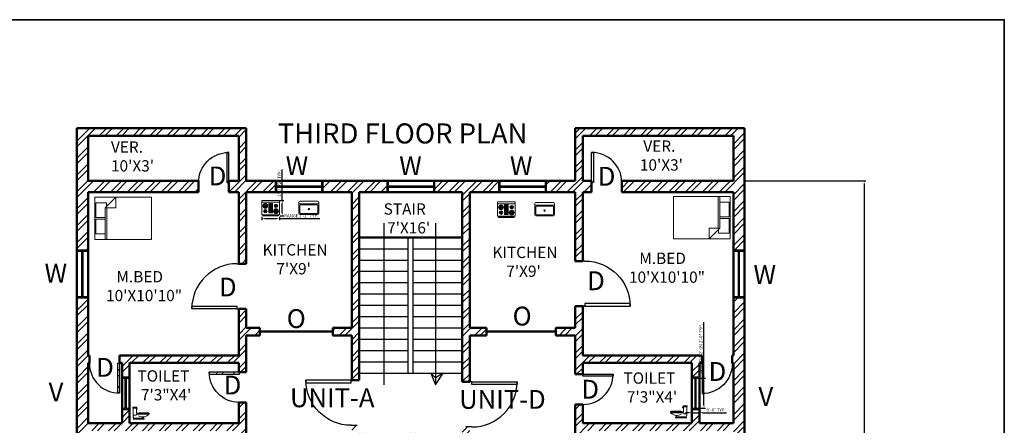
# Model space of a CAD drawing. Units: inches. Extents: x -31842 to -29388, y 18869 to 19743.
# Tile 12 of 12: x -30172 to -29388, y 19420 to 19743. Entities that reach past the tile are written whole.
import ezdxf

# ---------------------------------------------------------------- set-up
doc = ezdxf.new("R2010")
doc.units = ezdxf.units.IN
for name, color, linetype, lineweight in [('A-ANNO-DIMS', 2, 'Continuous', 18), ('A-ANNO-SYMB', 2, 'Continuous', 18), ('A-ANNO-TEXT', 7, 'Continuous', 25), ('A-ANNO-TTLB', 7, 'Continuous', 35), ('A-AREA-IDEN', 3, 'Continuous', 18), ('A-DOOR', 3, 'Continuous', 25), ('A-FLOR-FIXT', 8, 'Continuous', 18), ('A-FLOR-STRS', 7, 'Continuous', 25), ('A-FURN', 8, 'Continuous', 18), ('A-GLAZ', 4, 'Continuous', 25), ('A-WALL', 7, 'Continuous', 50), ('A-WALL-PATT', 8, 'Continuous', 13)]:
    doc.layers.add(name, color=color, linetype=linetype, lineweight=lineweight)
doc.styles.get("Standard").update_dxf_attribs({"font": 'arial.ttf'})
doc.dimstyles.new('ISO-25', dxfattribs={"dimtxt": 2.5, "dimasz": 2.5, "dimexe": 1.25, "dimexo": 0.625, "dimtad": 1, "dimdec": 0, "dimlunit": 3, "dimtxsty": 'Standard', "dimcen": 2.5, "dimadec": 0, "dimazin": 0, "dimtfac": 1, "dimtdec": 0, "dimtmove": 0, "dimatfit": 3, "dimfxl": 1, "dimarcsym": 0})

# ---------------------------------------------------------------- blocks, each defined once
blk = doc.blocks.new('*U8')
for p, q in [((0, 0), (0, -100)), ((750, 0), (750, -100))]:
    blk.add_line(p, q)
blk.add_lwpolyline([(0, 0), (0, 750), (43.75, 750), (43.75, 0)], close=True)
blk.add_arc((0, 0), 750, 0, 90)
blk = doc.blocks.new('Bed - Queen')
for p, q in [((0, -80.00003), (0, 0)), ((0, 0), (59.99999, 0)), ((59.99999, 0), (59.99999, -80.00003)), ((7.99999, -1.2), (28.79998, -1.2)), ((7.99999, -14.4), (7.99999, -1.2)), ((28.79998, -1.2), (28.79998, -14.4)), ((31.19999, -1.2), (51.99999, -1.2)), ((31.19999, -14.4), (31.19999, -1.2)), ((51.99999, -1.2), (51.99999, -16.4)), ((0, -14.4), (44.8, -14.4)), ((44.8, -16.8), (0, -16.8)), ((59.99999, -29.6), (44.8, -14.4)), ((44.8, -14.4), (44.8, -29.6)), ((51.99999, -16.4), (46.79936, -16.4)), ((44.8, -29.6), (59.99999, -29.6)), ((59.99999, -80.00003), (0, -80.00003))]:
    blk.add_line(p, q)
blk = doc.blocks.new('Range-Oven - 30 in top')
for p, q in [((0, -3), (30, -3)), ((12, -6), (18, -6)), ((13, -20), (13, -6)), ((14, -6), (14, -20)), ((15, -20), (15, -6)), ((16, -6), (16, -20)), ((17, -20), (17, -6)), ((6, -24), (6, -25)), ((8, -25), (8, -24)), ((18, -20), (12, -20)), ((22, -25), (22, -24)), ((24, -24), (24, -25))]:
    blk.add_line(p, q)
for points in [[(0, -24), (0, 0), (30, 0), (30, -24)], [(12, -21), (12, -5), (18, -5), (18, -21)], [(2, -26), (2, -25), (28, -25), (28, -26)]]:
    blk.add_lwpolyline(points, close=True)
for centre, radius in [((6, -9), 4), ((6, -9), 3), ((6, -18), 3), ((6, -9), 2), ((6, -18), 2), ((6, -9), 1), ((24, -18), 4), ((24, -9), 3), ((24, -18), 3), ((24, -9), 2), ((24, -18), 2), ((24, -9), 1), ((6, -18), 1), ((24, -18), 1)]:
    blk.add_circle(centre, radius)
blk = doc.blocks.new('Sink-single - 30 in top')
blk.add_line((-15, -3.999996), (15, -3.999996))
for points in [[(-13.5, 0), (13.5, 0)], [(-15, -18.499996), (-15, -1.5)], [(-13.5, -17.499996), (-13.5, -6.499996)], [(-12.5, -5.499996), (12.5, -5.499996)], [(13.5, -6.499996), (13.5, -17.499996)], [(15, -1.5), (15, -18.499996)], [(13.5, -19.999996), (-13.5, -19.999996)], [(12.5, -18.499996), (-12.5, -18.499996)]]:
    blk.add_lwpolyline(points)
for radius in [1, 0.5]:
    blk.add_circle((0, -11.999996), radius)
for centre, radius, start, end in [((-13.5, -1.5), 1.5, 90, 180), ((-12.5, -6.499996), 1, 90, 180), ((12.5, -6.499996), 1, 0, 90), ((13.5, -1.5), 1.5, 0, 90), ((-13.5, -18.499996), 1.5, 180, 270), ((-12.5, -17.499996), 1, 180, 270), ((12.5, -17.499996), 1, 270, 0), ((13.5, -18.499996), 1.5, 270, 0)]:
    blk.add_arc(centre, radius, start, end)
blk = doc.blocks.new('Toilet - side')
for p, q in [((0.5, 5), (0.5, 22)), ((7.5, 22), (7.5, 12)), ((7.5, 21), (9, 21)), ((9, 20), (7.5, 20)), ((9, 21), (9, 20)), ((6, 8), (0.5, 8)), ((22, 2), (2, 2)), ((2, 2), (2, 1)), ((8, 10), (6, 8)), ((7.5, 12), (33, 12)), ((33, 10), (8, 10)), ((32.5, 13), (12, 13)), ((12, 13), (12, 12)), ((21, 4.5), (21, 2)), ((22, 2), (22, 4.5)), ((22, 1), (22, 2)), ((32.5, 12), (32.5, 13)), ((33, 12), (33, 10))]:
    blk.add_line(p, q)
for points in [[(0, 22), (0, 24), (8, 24), (8, 22)], [(1, 0), (1, 1), (23, 1), (23, 0)]]:
    blk.add_lwpolyline(points, close=True)
for centre, radius, start, end in [((3.8, 4.8), 3.26, 175.6013, 237.5288), ((20.3, 20.7), 16.2, 238.1872, 318.7702)]:
    blk.add_arc(centre, radius, start, end)
blk = doc.blocks.new('*D211')
at = {"layer": 'A-ANNO-DIMS', "color": 0, "lineweight": -2, "transparency": 16777216}
for p, q in [((-29593.87, 19614.96), (-29498.06, 19614.96)), ((-29499.31, 19612.46), (-29499.31, 19017.46)), ((-29593.87, 19014.96), (-29498.06, 19014.96))]:
    blk.add_line(p, q, dxfattribs=at)
at = {"layer": 'A-ANNO-DIMS', "color": 0, "transparency": 16777216}
for points in [[(-29499.72, 19612.46), (-29498.89, 19612.46), (-29499.31, 19614.96)], [(-29499.72, 19017.46), (-29498.89, 19017.46), (-29499.31, 19014.96)]]:
    blk.add_solid(points, dxfattribs=at)
at = {"layer": 'Defpoints', "color": 0, "transparency": 16777216}
for p in [(-29594.5, 19614.96), (-29594.5, 19014.96), (-29499.31, 19014.96)]:
    blk.add_point(p, dxfattribs=at)
at = {"layer": 'A-ANNO-DIMS', "color": 0, "transparency": 16777216, "insert": (-29508.1, 19314.96), "char_height": 2.5, "attachment_point": 5, "rotation": 90}
blk.add_mtext("{\\H6.4x;50'}", dxfattribs=at)
blk = doc.blocks.new('WIN-3FT')
for p, q in [((0, 36), (9, 36)), ((4, 0), (4, 36)), ((4.5, 0), (4.5, 36)), ((5, 0), (5, 36)), ((0, 0), (9, 0))]:
    blk.add_line(p, q)
blk = doc.blocks.new('WIN-2FT-B')
for p, q in [((0, 24), (6, 24)), ((2.5, 0), (2.5, 24)), ((3, 0), (3, 24)), ((3.5, 0), (3.5, 24)), ((0, 0), (6, 0))]:
    blk.add_line(p, q)
blk = doc.blocks.new('*D235')
at = {"layer": 'A-ANNO-DIMS', "color": 0, "lineweight": -2, "transparency": 16777216}
for p, q in [((-29979.2, 19586.46), (-29979.2, 19583.71)), ((-29965.04, 19586.46), (-29965.04, 19583.71)), ((-29976.7, 19584.96), (-29967.54, 19584.96)), ((-29965.04, 19584.96), (-29932.79, 19584.96))]:
    blk.add_line(p, q, dxfattribs=at)
at = {"layer": 'A-ANNO-DIMS', "color": 0, "transparency": 16777216}
for points in [[(-29976.7, 19585.38), (-29976.7, 19584.54), (-29979.2, 19584.96)], [(-29967.54, 19585.38), (-29967.54, 19584.54), (-29965.04, 19584.96)]]:
    blk.add_solid(points, dxfattribs=at)
at = {"layer": 'Defpoints', "color": 0, "transparency": 16777216}
for p in [(-29979.2, 19587.08), (-29965.04, 19587.08), (-29965.04, 19584.96)]:
    blk.add_point(p, dxfattribs=at)
at = {"layer": 'A-ANNO-DIMS', "color": 0, "transparency": 16777216, "insert": (-29947.66, 19586.88), "char_height": 2.5, "attachment_point": 5}
blk.add_mtext('RANGE 1\'-2" TYP.', dxfattribs=at)
blk = doc.blocks.new('*D236')
at = {"layer": 'A-ANNO-DIMS', "color": 0, "lineweight": -2, "transparency": 16777216}
for p, q in [((-29962.91, 19599.36), (-29962.91, 19623.94)), ((-29964.41, 19599.36), (-29961.66, 19599.36)), ((-29962.91, 19589.58), (-29962.91, 19596.86)), ((-29964.41, 19587.08), (-29961.66, 19587.08))]:
    blk.add_line(p, q, dxfattribs=at)
at = {"layer": 'A-ANNO-DIMS', "color": 0, "transparency": 16777216}
for points in [[(-29963.33, 19596.86), (-29962.49, 19596.86), (-29962.91, 19599.36)], [(-29963.33, 19589.58), (-29962.49, 19589.58), (-29962.91, 19587.08)]]:
    blk.add_solid(points, dxfattribs=at)
at = {"layer": 'Defpoints', "color": 0, "transparency": 16777216}
for p in [(-29965.04, 19599.36), (-29962.91, 19599.36), (-29965.04, 19587.08)]:
    blk.add_point(p, dxfattribs=at)
at = {"layer": 'A-ANNO-DIMS', "color": 0, "transparency": 16777216, "insert": (-29964.83, 19612.9), "char_height": 2.5, "attachment_point": 5, "rotation": 90}
blk.add_mtext('1\'-0 1/2" TYP.', dxfattribs=at)
blk = doc.blocks.new('*D261')
at = {"layer": 'A-ANNO-DIMS', "color": 0, "lineweight": -2, "transparency": 16777216}
for p, q in [((-29626.9, 19457.96), (-29626.9, 19502.55)), ((-29629.87, 19457.96), (-29625.65, 19457.96)), ((-29626.9, 19436.46), (-29626.9, 19455.46)), ((-29629.87, 19433.96), (-29625.65, 19433.96))]:
    blk.add_line(p, q, dxfattribs=at)
at = {"layer": 'A-ANNO-DIMS', "color": 0, "transparency": 16777216}
for points in [[(-29627.31, 19455.46), (-29626.48, 19455.46), (-29626.9, 19457.96)], [(-29627.31, 19436.46), (-29626.48, 19436.46), (-29626.9, 19433.96)]]:
    blk.add_solid(points, dxfattribs=at)
at = {"layer": 'Defpoints', "color": 0, "transparency": 16777216}
for p in [(-29630.5, 19457.96), (-29626.9, 19457.96), (-29630.5, 19433.96)]:
    blk.add_point(p, dxfattribs=at)
at = {"layer": 'A-ANNO-DIMS', "color": 0, "transparency": 16777216, "insert": (-29629.16, 19481.51), "char_height": 2.5, "attachment_point": 5, "rotation": 90}
blk.add_mtext('WINDOW 2\' (B) 2\'-0" TYP.', dxfattribs=at)
blk = doc.blocks.new('*D262')
at = {"layer": 'A-ANNO-DIMS', "color": 0, "lineweight": -2, "transparency": 16777216}
for p, q in [((-29639, 19430.36), (-29641.5, 19430.36)), ((-29636.5, 19433.34), (-29636.5, 19429.11)), ((-29636.5, 19430.36), (-29630.5, 19430.36)), ((-29630.5, 19433.34), (-29630.5, 19429.11)), ((-29628, 19430.36), (-29609.01, 19430.36))]:
    blk.add_line(p, q, dxfattribs=at)
at = {"layer": 'A-ANNO-DIMS', "color": 0, "transparency": 16777216}
for points in [[(-29639, 19430.78), (-29639, 19429.94), (-29636.5, 19430.36)], [(-29628, 19430.78), (-29628, 19429.94), (-29630.5, 19430.36)]]:
    blk.add_solid(points, dxfattribs=at)
at = {"layer": 'Defpoints', "color": 0, "transparency": 16777216}
for p in [(-29636.5, 19433.96), (-29630.5, 19433.96), (-29630.5, 19430.36)]:
    blk.add_point(p, dxfattribs=at)
at = {"layer": 'A-ANNO-DIMS', "color": 0, "transparency": 16777216, "insert": (-29617.25, 19432.26), "char_height": 2.5, "attachment_point": 5}
blk.add_mtext('0\'-6" TYP.', dxfattribs=at)

msp = doc.modelspace()

# ---------------------------------------------------------------- hatches: boundary and pattern name
at = {"layer": 'A-WALL-PATT'}
h = msp.add_hatch(dxfattribs=at)
h.set_pattern_fill('ANSI32', color=256)
h.paths.add_polyline_path([(-29790.5, 19614.96), (-29841.5, 19614.96), (-29841.5, 19605.96), (-29819.5, 19605.96), (-29819.5, 19455.01), (-29813.5, 19455.01), (-29813.5, 19491.96), (-29800.11, 19491.96), (-29800.11, 19497.96), (-29813.5, 19497.96), (-29813.5, 19605.96), (-29790.5, 19605.96)])
h.paths.add_polyline_path([(-29879.5, 19614.96), (-29930.5, 19614.96), (-29930.5, 19605.96), (-29907.5, 19605.96), (-29907.5, 19497.96), (-29922.61, 19497.96), (-29922.61, 19491.96), (-29907.5, 19491.96), (-29907.5, 19456.33), (-29903.21, 19456.33), (-29901.5, 19456.31), (-29901.5, 19605.96), (-29879.5, 19605.96)])
h.paths.add_polyline_path([(-29968.5, 19614.96), (-29991.5, 19614.96), (-29991.5, 19656.96), (-30126.5, 19656.96), (-30126.5, 19559.96), (-30117.5, 19559.96), (-30117.5, 19605.96), (-30029.48, 19605.96), (-30029.48, 19614.96), (-30117.5, 19614.96), (-30117.5, 19650.96), (-29997.5, 19650.96), (-29997.5, 19614.96), (-30005.48, 19614.96), (-30005.48, 19605.96), (-29997.5, 19605.96), (-29997.5, 19549.04), (-29991.5, 19549.04), (-29991.5, 19605.96), (-29968.5, 19605.96)])
h.paths.add_polyline_path([(-29716.42, 19614.96), (-29723.5, 19614.96), (-29723.5, 19650.96), (-29603.5, 19650.96), (-29603.5, 19614.96), (-29692.42, 19614.96), (-29692.42, 19605.96), (-29687.14, 19605.96), (-29603.5, 19605.96), (-29603.5, 19559.96), (-29594.5, 19559.96), (-29594.5, 19656.96), (-29729.5, 19656.96), (-29729.5, 19614.96), (-29752.5, 19614.96), (-29752.5, 19605.96), (-29729.5, 19605.96), (-29729.5, 19551.13), (-29723.5, 19551.13), (-29723.5, 19605.96), (-29716.42, 19605.96)])
h.paths.add_polyline_path([(-29628.39, 19472.82), (-29628.34, 19475.96), (-29723.5, 19475.96), (-29723.5, 19515.13), (-29729.5, 19515.13), (-29729.5, 19497.96), (-29744.93, 19497.96), (-29744.93, 19491.96), (-29729.5, 19491.96), (-29729.5, 19460.98), (-29723.5, 19460.98), (-29723.5, 19469.96), (-29636.5, 19469.96), (-29636.5, 19458.96), (-29630.5, 19458.96), (-29630.5, 19469.96), (-29628.39, 19469.96)])
h.paths.add_polyline_path([(-29594.5, 19521.96), (-29603.5, 19521.96), (-29603.5, 19475.96), (-29604.34, 19475.96), (-29604.34, 19469.96), (-29603.5, 19469.96), (-29603.5, 19421.96), (-29630.5, 19421.96), (-29630.5, 19432.96), (-29636.5, 19432.96), (-29636.5, 19421.96), (-29723.5, 19421.96), (-29723.5, 19436.98), (-29729.5, 19436.98), (-29729.5, 19396.75), (-29723.5, 19396.75), (-29723.5, 19415.96), (-29603.5, 19415.96), (-29603.5, 19369.96), (-29594.5, 19369.96)])
h.paths.add_polyline_path([(-29594.5, 19331.96), (-29603.5, 19331.96), (-29603.5, 19285.96), (-29723.5, 19285.96), (-29723.5, 19360.75), (-29729.5, 19360.75), (-29729.5, 19285.96), (-29813.5, 19285.96), (-29813.5, 19419.01), (-29819.5, 19419.01), (-29819.5, 19413.96), (-29825.38, 19413.96), (-29825.38, 19407.96), (-29819.5, 19407.96), (-29819.5, 19279.96), (-29688.5, 19279.96), (-29688.5, 19267.87), (-29682.5, 19267.87), (-29682.5, 19279.96), (-29603.5, 19279.96), (-29603.5, 19262.96), (-29594.5, 19262.96)])
h.paths.add_polyline_path([(-29594.5, 19224.96), (-29603.5, 19224.96), (-29603.5, 19207.96), (-29682.5, 19207.96), (-29682.5, 19219.98), (-29688.5, 19219.98), (-29688.5, 19194.76), (-29682.5, 19194.76), (-29682.5, 19201.96), (-29603.5, 19201.96), (-29603.5, 19190.96), (-29594.5, 19190.96)])
h.paths.add_polyline_path([(-29564.5, 19153.96), (-29584.31, 19153.96), (-29584.31, 19147.96), (-29570.5, 19147.96), (-29570.5, 19023.96), (-29615.5, 19023.96), (-29615.5, 19066.96), (-29621.5, 19066.96), (-29621.5, 19023.96), (-29653.5, 19023.96), (-29653.5, 19014.96), (-29564.5, 19014.96)])
h.paths.add_polyline_path([(-29608.31, 19153.96), (-29682.5, 19153.96), (-29682.5, 19170.76), (-29688.5, 19170.76), (-29688.5, 19153.96), (-29691.71, 19153.96), (-29691.71, 19147.96), (-29621.5, 19147.96), (-29621.5, 19104.96), (-29615.5, 19104.96), (-29615.5, 19147.96), (-29608.31, 19147.96)])
h.paths.add_polyline_path([(-29721.71, 19153.96), (-29739.81, 19153.96), (-29739.81, 19147.96), (-29729.5, 19147.96), (-29729.5, 19023.96), (-29774, 19023.96), (-29774, 19014.96), (-29691.5, 19014.96), (-29691.5, 19023.96), (-29723.5, 19023.96), (-29723.5, 19147.96), (-29721.71, 19147.96)])
h.paths.add_polyline_path([(-29946, 19023.96), (-29991.5, 19023.96), (-29991.5, 19147.96), (-29988.28, 19147.96), (-29988.28, 19153.96), (-30000.21, 19153.96), (-30000.21, 19147.96), (-29997.5, 19147.96), (-29997.5, 19023.96), (-30029.5, 19023.96), (-30029.5, 19014.96), (-29946, 19014.96)])
h.paths.add_polyline_path([(-30067.5, 19023.96), (-30099.5, 19023.96), (-30099.5, 19066.96), (-30105.5, 19066.96), (-30105.5, 19023.96), (-30150.5, 19023.96), (-30150.5, 19147.96), (-30137.18, 19147.96), (-30137.18, 19153.96), (-30156.5, 19153.96), (-30156.5, 19014.96), (-30067.5, 19014.96)])
h.paths.add_polyline_path([(-30099.5, 19147.96), (-30030.21, 19147.96), (-30030.21, 19153.96), (-30032.5, 19153.96), (-30032.5, 19173.83), (-30038.5, 19173.83), (-30038.5, 19153.96), (-30113.18, 19153.96), (-30113.18, 19147.96), (-30105.5, 19147.96), (-30105.5, 19104.96), (-30099.5, 19104.96)])
h.paths.add_polyline_path([(-30032.5, 19217.89), (-30038.5, 19217.89), (-30038.5, 19207.96), (-30117.5, 19207.96), (-30117.5, 19224.96), (-30126.5, 19224.96), (-30126.5, 19190.96), (-30117.5, 19190.96), (-30117.5, 19201.96), (-30038.5, 19201.96), (-30038.5, 19197.83), (-30032.5, 19197.83)])
h.paths.add_polyline_path([(-29901.5, 19407.96), (-29893.72, 19407.96), (-29893.72, 19413.96), (-29901.5, 19413.96), (-29901.5, 19420.31), (-29907.5, 19420.31), (-29907.5, 19285.96), (-29991.5, 19285.96), (-29991.5, 19365.01), (-29997.5, 19365.01), (-29997.5, 19285.96), (-30117.5, 19285.96), (-30117.5, 19331.96), (-30126.5, 19331.96), (-30126.5, 19262.96), (-30117.5, 19262.96), (-30117.5, 19279.96), (-30038.5, 19279.96), (-30038.5, 19268.29), (-30032.5, 19268.29), (-30032.5, 19279.96), (-29901.5, 19279.96)])
h.paths.add_polyline_path([(-29863.72, 19413.96), (-29855.38, 19413.96), (-29855.38, 19406.96), (-29853.63, 19406.96), (-29853.63, 19376.96), (-29856.5, 19376.96), (-29856.5, 19153.96), (-29775.81, 19153.96), (-29775.81, 19148.44, 0.39722), (-29741.97, 19112.57), (-29741.97, 19148.44), (-29739.88, 19148.44), (-29739.88, 19112.51), (-29741.97, 19112.51), (-29741.97, 19112.57, -0.393359), (-29775.8, 19147.96), (-29856.5, 19147.96), (-29856.5, 19023.96), (-29811, 19023.96), (-29811, 19014.96), (-29909, 19014.96), (-29909, 19018.96), (-29945, 19018.96), (-29945, 19019.96), (-29909, 19019.96), (-29909, 19023.96), (-29862.5, 19023.96), (-29862.5, 19147.96), (-29901.5, 19147.96), (-29952.22, 19147.96), (-29952.22, 19146.6, -0.39722), (-29986.12, 19110.67), (-29986.12, 19110.6), (-29988.22, 19110.6), (-29988.22, 19146.6), (-29986.12, 19146.6), (-29986.12, 19110.67, 0.39722), (-29952.22, 19146.6), (-29952.22, 19147.96), (-29952.28, 19147.96), (-29952.28, 19153.96), (-29901.5, 19153.96), (-29862.5, 19153.96), (-29862.5, 19407.96), (-29863.72, 19407.96), (-29863.72, 19406.62), (-29863.72, 19376.63), (-29865.47, 19376.63), (-29865.47, 19406.62), (-29863.72, 19406.62), (-29863.72, 19407.96), (-29863.72, 19407.96)])
h.paths.add_polyline_path([(-30021.02, 19461.17), (-30021.06, 19461.17), (-30021.06, 19462.57), (-29997.02, 19462.57), (-29997.02, 19461.17), (-30021.02, 19461.17, 0.386026), (-29997.95, 19438.55), (-29991.5, 19438.55), (-29991.5, 19401.01), (-29998.66, 19401.01), (-29998.66, 19398.9), (-30034.72, 19398.9), (-30034.72, 19401.01), (-29997.5, 19401.01), (-29997.5, 19415.96), (-30117.5, 19415.96), (-30117.5, 19368.96), (-30121.5, 19368.96), (-30121.5, 19332.96), (-30122.5, 19332.96), (-30122.5, 19368.96), (-30126.5, 19368.96), (-30126.5, 19522.96), (-30117.5, 19522.96), (-30117.5, 19475.96), (-30116.52, 19475.96), (-30116.52, 19469.92, 0.39722), (-30093.92, 19445.96), (-30093.92, 19469.92), (-30092.52, 19469.92), (-30092.52, 19445.92), (-30093.92, 19445.92), (-30093.92, 19445.96, -0.39722), (-30116.52, 19469.92), (-30117.5, 19421.96), (-30090.5, 19421.96), (-30090.5, 19433.96), (-30084.5, 19433.96), (-30084.5, 19421.96), (-29997.5, 19421.96), (-29997.5, 19438.54, -0.391477)])
h.paths.add_polyline_path([(-29991.5, 19491.96), (-29980.66, 19491.96), (-29980.66, 19497.96), (-29991.5, 19497.96), (-29991.5, 19513.04), (-29997.5, 19513.04), (-29997.5, 19475.96), (-30092.52, 19475.96), (-30092.52, 19469.96), (-30090.5, 19469.96), (-30090.5, 19458.96), (-30084.5, 19458.96), (-30084.5, 19469.96), (-29997.5, 19469.96), (-29997.5, 19462.57), (-29997.02, 19462.57), (-29991.5, 19462.55)])
h.paths.add_polyline_path([(-29857.76, 19352.86), (-29815.8, 19352.86), (-29815.8, 19369.38), (-29857.76, 19369.38)], flags=24)

# ---------------------------------------------------------------- linework, layer by layer
at = {"layer": 'A-ANNO-TTLB'}
msp.add_lwpolyline([(-31842.18, 19743.36), (-29387.67, 19743.36), (-29387.67, 18868.82), (-31842.18, 18868.82)], close=True, dxfattribs=at)
at = {"layer": 'A-FLOR-STRS'}
for p, q in [((-29882, 19581.21), (-29882, 19452.66)), ((-29840.68, 19581.21), (-29840.68, 19452.66)), ((-29862.5, 19461.96), (-29862.5, 19569.96)), ((-29858.5, 19461.96), (-29858.5, 19569.96)), ((-29901.5, 19560.96), (-29862.5, 19560.96)), ((-29858.5, 19560.96), (-29819.5, 19560.96)), ((-29901.5, 19551.96), (-29862.5, 19551.96)), ((-29858.5, 19551.96), (-29819.5, 19551.96)), ((-29901.5, 19542.96), (-29862.5, 19542.96)), ((-29858.5, 19542.96), (-29819.5, 19542.96)), ((-29901.5, 19533.96), (-29862.5, 19533.96)), ((-29858.5, 19533.96), (-29819.5, 19533.96)), ((-29901.5, 19524.96), (-29862.5, 19524.96)), ((-29858.5, 19524.96), (-29819.5, 19524.96)), ((-29901.5, 19515.96), (-29862.5, 19515.96)), ((-29858.5, 19515.96), (-29819.5, 19515.96)), ((-29901.5, 19506.96), (-29862.5, 19506.96)), ((-29858.5, 19506.96), (-29819.5, 19506.96)), ((-29901.5, 19497.96), (-29862.5, 19497.96)), ((-29858.5, 19497.96), (-29819.5, 19497.96)), ((-29901.5, 19488.96), (-29862.5, 19488.96)), ((-29858.5, 19488.96), (-29819.5, 19488.96)), ((-29901.5, 19479.96), (-29862.5, 19479.96)), ((-29858.5, 19479.96), (-29819.5, 19479.96)), ((-29901.5, 19470.96), (-29862.5, 19470.96)), ((-29858.5, 19470.96), (-29819.5, 19470.96)), ((-29901.5, 19461.96), (-29819.5, 19461.96)), ((-29840.68, 19458.24), (-29844.38, 19461.96)), ((-29844.38, 19461.96), (-29840.68, 19452.66)), ((-29840.68, 19452.66), (-29834.65, 19461.96)), ((-29834.65, 19461.96), (-29840.68, 19458.24))]:
    msp.add_line(p, q, dxfattribs=at)
at = {"layer": 'A-GLAZ'}
for p, q in [((-29968.5, 19614.96), (-29968.5, 19605.96)), ((-29930.5, 19614.96), (-29930.5, 19605.96)), ((-29879.5, 19614.96), (-29879.5, 19605.96)), ((-29841.5, 19614.96), (-29841.5, 19605.96)), ((-29790.5, 19614.96), (-29790.5, 19605.96)), ((-29752.5, 19614.96), (-29752.5, 19605.96)), ((-30126.5, 19559.96), (-30117.5, 19559.96)), ((-29603.5, 19559.96), (-29594.5, 19559.96)), ((-30126.5, 19521.96), (-30117.5, 19521.96)), ((-29603.5, 19521.96), (-29594.5, 19521.96)), ((-30090.5, 19458.96), (-30084.5, 19458.96)), ((-29636.5, 19458.96), (-29630.5, 19458.96)), ((-30090.5, 19432.96), (-30084.5, 19432.96)), ((-29636.5, 19432.96), (-29630.5, 19432.96))]:
    msp.add_line(p, q, dxfattribs=at)
at = {"layer": 'A-WALL'}
for p, q in [((-30126.5, 19153.96), (-30126.5, 19656.96)), ((-30126.5, 19656.96), (-29991.5, 19656.96)), ((-29991.5, 19614.96), (-29991.5, 19656.96)), ((-29729.5, 19656.96), (-29729.5, 19614.96)), ((-29729.5, 19656.96), (-29594.5, 19656.96)), ((-29594.5, 19656.96), (-29594.5, 19153.96)), ((-30117.5, 19650.96), (-29997.5, 19650.96)), ((-30117.5, 19614.96), (-30117.5, 19650.96)), ((-29997.5, 19614.96), (-29997.5, 19650.96)), ((-29723.5, 19650.96), (-29723.5, 19614.96)), ((-29723.5, 19650.96), (-29603.5, 19650.96)), ((-29603.5, 19650.96), (-29603.5, 19614.96)), ((-30117.5, 19614.96), (-30029.48, 19614.96)), ((-30029.48, 19614.96), (-30029.48, 19605.96)), ((-30005.48, 19614.96), (-30005.48, 19605.96)), ((-30005.48, 19614.96), (-29997.5, 19614.96)), ((-29991.5, 19614.96), (-29729.5, 19614.96)), ((-29723.5, 19614.96), (-29716.42, 19614.96)), ((-29716.42, 19614.96), (-29716.42, 19605.96)), ((-29692.42, 19614.96), (-29692.42, 19605.96)), ((-29692.42, 19614.96), (-29603.5, 19614.96)), ((-30117.5, 19605.96), (-30029.48, 19605.96)), ((-30117.5, 19475.96), (-30117.5, 19605.96)), ((-30005.48, 19605.96), (-29997.5, 19605.96)), ((-29997.5, 19549.04), (-29997.5, 19605.96)), ((-29991.5, 19605.96), (-29907.5, 19605.96)), ((-29991.5, 19549.04), (-29991.5, 19605.96)), ((-29907.5, 19497.96), (-29907.5, 19605.96)), ((-29901.5, 19605.96), (-29819.5, 19605.96)), ((-29901.5, 19456.31), (-29901.5, 19605.96)), ((-29819.5, 19605.96), (-29819.5, 19455.01)), ((-29813.5, 19605.96), (-29813.5, 19497.96)), ((-29813.5, 19605.96), (-29729.5, 19605.96)), ((-29729.5, 19605.96), (-29729.5, 19551.13)), ((-29723.5, 19605.96), (-29723.5, 19551.13)), ((-29723.5, 19605.96), (-29716.42, 19605.96)), ((-29692.42, 19605.96), (-29687.14, 19605.96)), ((-29692.42, 19605.96), (-29603.5, 19605.96)), ((-29603.5, 19605.96), (-29603.5, 19475.96)), ((-29901.5, 19569.96), (-29819.5, 19569.96)), ((-29997.5, 19549.04), (-29991.5, 19549.04)), ((-29729.5, 19551.13), (-29723.5, 19551.13)), ((-29729.5, 19515.13), (-29723.5, 19515.13)), ((-29729.5, 19515.13), (-29729.5, 19497.96)), ((-29723.5, 19515.13), (-29723.5, 19475.96)), ((-29997.5, 19475.96), (-29997.5, 19513.04)), ((-29997.5, 19513.04), (-29991.5, 19513.04)), ((-29991.5, 19497.96), (-29991.5, 19513.04)), ((-29991.5, 19497.96), (-29980.66, 19497.96)), ((-29991.5, 19491.96), (-29980.66, 19491.96)), ((-29991.5, 19462.55), (-29991.5, 19491.96)), ((-29980.66, 19497.96), (-29980.66, 19491.96)), ((-29980.66, 19494.96), (-29922.61, 19494.96)), ((-29922.61, 19497.96), (-29922.61, 19491.96)), ((-29922.61, 19497.96), (-29907.5, 19497.96)), ((-29922.61, 19491.96), (-29907.5, 19491.96)), ((-29907.5, 19456.31), (-29907.5, 19491.96)), ((-29813.5, 19497.96), (-29800.11, 19497.96)), ((-29813.5, 19491.96), (-29800.11, 19491.96)), ((-29813.5, 19491.96), (-29813.5, 19455.01)), ((-29800.11, 19497.96), (-29800.11, 19491.96)), ((-29800.11, 19494.96), (-29744.93, 19494.96)), ((-29744.93, 19497.96), (-29744.93, 19491.96)), ((-29744.93, 19497.96), (-29729.5, 19497.96)), ((-29744.93, 19491.96), (-29729.5, 19491.96)), ((-29729.5, 19491.96), (-29729.5, 19460.98)), ((-30117.5, 19475.96), (-30116.52, 19475.96)), ((-30116.52, 19469.96), (-30116.52, 19475.96)), ((-30092.52, 19469.96), (-30092.52, 19475.96)), ((-30092.52, 19475.96), (-29997.5, 19475.96)), ((-29723.5, 19475.96), (-29628.34, 19475.96)), ((-29628.34, 19469.96), (-29628.34, 19475.96)), ((-29604.34, 19469.96), (-29604.34, 19475.96)), ((-29604.34, 19475.96), (-29603.5, 19475.96)), ((-30117.5, 19469.96), (-30116.52, 19469.96)), ((-30117.5, 19421.96), (-30117.5, 19469.96)), ((-30092.52, 19469.96), (-30090.5, 19469.96)), ((-30090.5, 19421.96), (-30090.5, 19469.96)), ((-30084.5, 19421.96), (-30084.5, 19469.96)), ((-30084.5, 19469.96), (-29997.5, 19469.96)), ((-29997.5, 19462.55), (-29997.5, 19469.96)), ((-29723.5, 19469.96), (-29636.5, 19469.96)), ((-29723.5, 19469.96), (-29723.5, 19460.98)), ((-29636.5, 19469.96), (-29636.5, 19421.96)), ((-29630.5, 19469.96), (-29630.5, 19421.96)), ((-29630.5, 19469.96), (-29628.34, 19469.96)), ((-29604.34, 19469.96), (-29603.5, 19469.96)), ((-29603.5, 19469.96), (-29603.5, 19421.96)), ((-29997.5, 19462.55), (-29991.5, 19462.55)), ((-29729.5, 19460.98), (-29723.5, 19460.98)), ((-29907.5, 19456.31), (-29901.5, 19456.31)), ((-29819.5, 19455.01), (-29813.5, 19455.01)), ((-29997.5, 19421.96), (-29997.5, 19438.55)), ((-29997.5, 19438.55), (-29991.5, 19438.55)), ((-29991.5, 19401.01), (-29991.5, 19438.55)), ((-29729.5, 19436.98), (-29723.5, 19436.98)), ((-29729.5, 19436.98), (-29729.5, 19396.75)), ((-29723.5, 19436.98), (-29723.5, 19421.96)), ((-30117.5, 19421.96), (-30090.5, 19421.96)), ((-30084.5, 19421.96), (-29997.5, 19421.96)), ((-29723.5, 19421.96), (-29636.5, 19421.96)), ((-29630.5, 19421.96), (-29603.5, 19421.96))]:
    msp.add_line(p, q, dxfattribs=at)

# ---------------------------------------------------------------- block references
at = {"layer": 'A-DOOR'}
for p, xscale, yscale, zscale in [((-30005.48, 19613.66), -0.0319999984510058, 0.0319999984510058, 0.0319999984510058), ((-29716.42, 19613.66), 0.0320000000000009, 0.0320000000000009, 0.0320000000000009)]:
    msp.add_blockref('*U8', p, dxfattribs=dict(at, xscale=xscale, yscale=yscale, zscale=zscale))
for p, xscale, yscale, zscale, rotation in [((-29998.94, 19513.04), 0.0479969271910708, 0.0479969271910708, 0.0479969271910708, 90.00000000000003), ((-29721.7, 19515.13), -0.0479999976070233, 0.0479999976070233, 0.0479999976070233, 270), ((-30092.52, 19469.92), 0.0320000000000009, 0.0320000000000009, 0.0320000000000009, 180), ((-29628.39, 19469.61), -0.0320770016506898, 0.0320770016506898, 0.0320770016506898, 180), ((-29997.02, 19462.57), -0.0320538111260468, 0.0320538111260468, 0.0320538111260468, 90), ((-29723.3, 19460.98), 0.0320000009996835, 0.0320000009996835, 0.0320000009996835, 270), ((-29908.01, 19456.33), -0.0480101042568555, 0.0480101042568555, 0.0480101042568555, 90), ((-29811.71, 19454.93), 0.0478936875771185, 0.0478936875771185, 0.0478936875771185, 270)]:
    msp.add_blockref('*U8', p, dxfattribs=dict(at, xscale=xscale, yscale=yscale, zscale=zscale, rotation=rotation))
at = {"layer": 'A-FLOR-FIXT'}
for name, p, xscale, yscale, zscale in [('Range-Oven - 30 in top', (-29979.2, 19599.36), 0.4722739601602511, 0.4722739601602511, 0.4722739601602511), ('Sink-single - 30 in top', (-29941.62, 19598.83), 0.526605956738203, 0.526605956738203, 0.526605956738203), ('Range-Oven - 30 in top', (-29791.43, 19598.21), 0.4722739601602511, 0.4722739601602511, 0.4722739601602511), ('Sink-single - 30 in top', (-29753.84, 19597.67), 0.526605956738203, 0.526605956738203, 0.526605956738203), ('Toilet - side', (-30081.9, 19425.18), 0.3964966977869737, 0.3964966977869737, 0.3964966977869737), ('Toilet - side', (-29640.36, 19426.35), -0.3964966977869737, 0.3964966977869737, 0.3964966977869737)]:
    msp.add_blockref(name, p, dxfattribs=dict(at, xscale=xscale, yscale=yscale, zscale=zscale))
at = {"layer": 'A-FURN', "xscale": 0.5638390730281776, "yscale": 0.5638390730281776, "zscale": 0.5638390730281776}
for p, rotation in [((-30112.09, 19568.2), 90), ((-29606.13, 19602.56), 270)]:
    msp.add_blockref('Bed - Queen', p, dxfattribs=dict(at, rotation=rotation))
at = {"layer": 'A-GLAZ', "rotation": 269.9999999999891}
for p in [(-29967.5, 19614.96), (-29878.5, 19614.96), (-29789.5, 19614.96)]:
    msp.add_blockref('WIN-3FT', p, dxfattribs=at)
at = {"layer": 'A-GLAZ'}
for name, p in [('WIN-3FT', (-30126.5, 19522.96)), ('WIN-3FT', (-29603.5, 19522.96)), ('WIN-2FT-B', (-30090.5, 19433.96)), ('WIN-2FT-B', (-29636.5, 19433.96))]:
    msp.add_blockref(name, p, dxfattribs=at)

# ---------------------------------------------------------------- texts
at = {"layer": 'A-ANNO-SYMB', "char_height": 15, "attachment_point": 1}
for s, insert in [('{W}', (-29960.13, 19634.55)), ('{W}', (-29869.69, 19634.55)), ('{W}', (-29781.52, 19634.55)), ('{D}', (-30021.43, 19626.42)), ('{D}', (-29711.5, 19626.15)), ('{W}', (-30152.22, 19548.99)), ('{W}', (-29587.48, 19547.87)), ('{D}', (-29719.97, 19542.94)), ('{D}', (-30013.28, 19537.94)), ('{O}', (-29779.35, 19514.79)), ('{O}', (-29959.3, 19512.8)), ('{D}', (-30111.07, 19473.94)), ('{D}', (-29623.25, 19470.67)), ('{D}', (-30009.52, 19459.88)), ('{V}', (-30148.98, 19454.3)), ('{D}', (-29724.58, 19456.53)), ('{V}', (-29583.52, 19450.8))]:
    msp.add_mtext_dynamic_manual_height_columns(s, width=1460.1328, gutter_width=12.5, heights=[0], dxfattribs=dict(at, insert=insert))
at = {"layer": 'A-ANNO-TEXT', "insert": (-29966.46, 19660.76), "char_height": 16, "attachment_point": 1}
msp.add_mtext_dynamic_manual_height_columns('{THIRD FLOOR PLAN}', width=1178.412, gutter_width=12.5, heights=[0], dxfattribs=at)
at = {"layer": 'A-AREA-IDEN', "attachment_point": 1}
for s, width, insert, char_height in [("{VER.\\P10'X3'}", 783.6296, (-30099.28, 19646.46), 9), ("{ VER.\\P10'X3'}", 783.6296, (-29677.96, 19647.18), 9), ("{   STAIR\\P    7'X16'}", 783.6296, (-29890.31, 19597.1), 9), ("{ KITCHEN\\P     7'X9'}", 783.6296, (-29981.28, 19564.54), 9), ("{KITCHEN\\P    7'X9'}", 783.6296, (-29795.4, 19562.52), 9), ('{   M.BED\\P10\'X10\'10"}', 783.6296, (-29686.66, 19557.8), 9), ('{   M.BED\\P10\'X10\'10"}', 783.6296, (-30103.22, 19543.17), 9), ('{TOILET\\P 7\'3"X4\'}', 783.6296, (-30078.18, 19464.12), 9), ('{   TOILET\\P    7\'3"X4\'}', 783.6296, (-29699.33, 19462.43), 9), ('{UNIT-A}', 1460.1328, (-29956.72, 19449.72), 15), ('{UNIT-D}', 1460.1328, (-29821.96, 19448.44), 15)]:
    msp.add_mtext_dynamic_manual_height_columns(s, width=width, gutter_width=12.5, heights=[0], dxfattribs=dict(at, insert=insert, char_height=char_height))

# ---------------------------------------------------------------- dimensions: what is measured, and where the dimension line sits
at = {"layer": 'A-ANNO-DIMS'}
for base, p1, p2, text, override, picture, middle in [((-29962.91, 19599.36), (-29965.04, 19587.08), (-29965.04, 19599.36), '<> TYP.', {"dimdec": 1, "dimlfac": 1, "dimrnd": 0, "dimzin": 1, "dimdsep": 46, "dimlunit": 4, "dimfrac": 2}, '*D236', (-29964.83, 19612.9)), ((-29499.31, 19014.96), (-29594.5, 19614.96), (-29594.5, 19014.96), '{\\H6.4x;<>}', {"dimclrd": 0, "dimclre": 0, "dimclrt": 0}, '*D211', (-29508.1, 19314.96)), ((-29626.9, 19457.96), (-29630.5, 19433.96), (-29630.5, 19457.96), "WINDOW 2' (B) <> TYP.", {"dimdec": 1, "dimlfac": 1, "dimrnd": 0, "dimzin": 1, "dimdsep": 46, "dimlunit": 4, "dimfrac": 2}, '*D261', (-29629.16, 19481.51))]:
    dim = msp.add_linear_dim(base=base, p1=p1, p2=p2, angle=90, text=text, dimstyle='ISO-25', override=override, dxfattribs=at)
    dim.commit()
    dim.dimension.update_dxf_attribs({"geometry": picture, "text_midpoint": middle})
for base, p1, p2, text, picture, middle in [((-29965.04, 19584.96), (-29979.2, 19587.08), (-29965.04, 19587.08), 'RANGE <> TYP.', '*D235', (-29947.66, 19586.88)), ((-29630.5, 19430.36), (-29636.5, 19433.96), (-29630.5, 19433.96), '<> TYP.', '*D262', (-29617.25, 19432.26))]:
    dim = msp.add_linear_dim(base=base, p1=p1, p2=p2, text=text, dimstyle='ISO-25', override={"dimdec": 1, "dimlfac": 1, "dimrnd": 0, "dimzin": 1, "dimdsep": 46, "dimlunit": 4, "dimfrac": 2}, dxfattribs=at)
    dim.commit()
    dim.dimension.update_dxf_attribs({"geometry": picture, "text_midpoint": middle})

doc.saveas('drawing.dxf')
